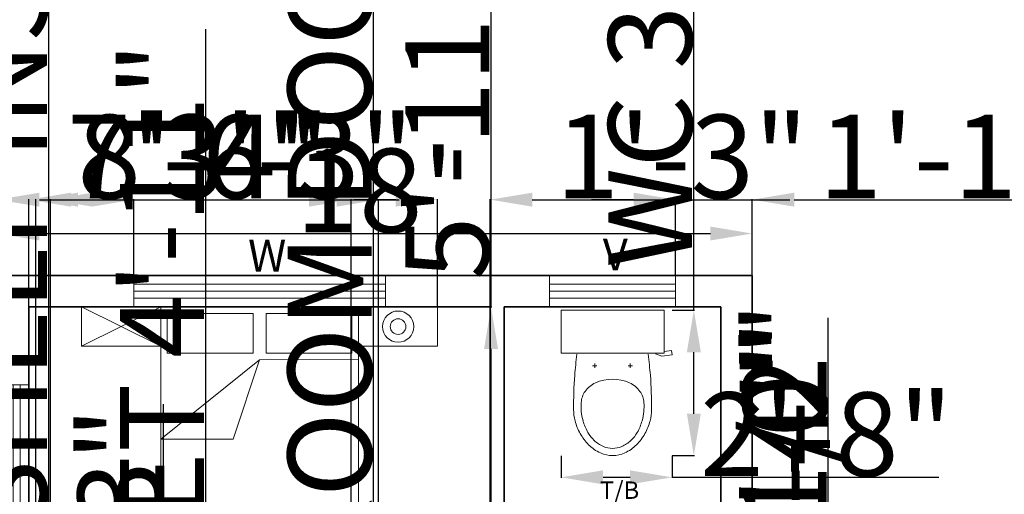
# Model space of a CAD drawing. Units: inches. Extents: x 2236 to 2927, y 1577 to 2452.
# Tile 7 of 9: x 2413 to 2695, y 2021 to 2157. Entities that reach past the tile are written whole.
import ezdxf

# ---------------------------------------------------------------- set-up
doc = ezdxf.new("R2010")
doc.units = ezdxf.units.IN
for name, color, linetype, lineweight in [('A-ANNO-DIMS', 2, 'Continuous', 18), ('A-ANNO-TEXT', 7, 'Continuous', 18), ('A-AREA-IDEN', 7, 'Continuous', 18), ('A-FLOR-FIXT', 9, 'Continuous', 18), ('A-FURN', 8, 'Continuous', 18), ('Wall', 7, 'Continuous', 35), ('Windows', 162, 'Continuous', 18)]:
    doc.layers.add(name, color=color, linetype=linetype, lineweight=lineweight)
doc.styles.get("Standard").update_dxf_attribs({"font": 'arial.ttf'})
doc.dimstyles.get("Standard").update_dxf_attribs({"dimtxt": 24, "dimasz": 12, "dimexe": 0.18, "dimexo": 0.0625, "dimgap": 0.09, "dimtad": 1, "dimdec": 1, "dimzin": 0, "dimdsep": 46, "dimlunit": 4, "dimtxsty": 'Standard', "dimcen": 0.09, "dimadec": 0, "dimazin": 0, "dimtfac": 1, "dimtdec": 1, "dimtofl": 0, "dimtmove": 0, "dimatfit": 3, "dimfxl": 1, "dimtolj": 1, "dimtzin": 0, "dimarcsym": 0})

# ---------------------------------------------------------------- blocks, each defined once
blk = doc.blocks.new('MAT-P13')
for p, q in [((-1.3496, 0), (-0.75, 0)), ((-1.3496, 0), (-1.3496, -0.2983)), ((-1.3496, -0.2983), (-0.75, 0)), ((-1.3496, 0), (-0.75, -0.2983)), ((-0.75, 0), (0.75, 0)), ((-0.75, 0), (-0.75, -1.9)), ((0.75, 0), (0.75, -1.9)), ((0.75, 0), (1.3496, 0)), ((1.3496, 0), (1.3496, -0.2983)), ((-0.7, -0.05), (-0.7, -0.35)), ((-0.7, -0.05), (-0.05, -0.05)), ((-0.05, -0.35), (-0.05, -0.05)), ((0.05, -0.05), (0.7, -0.05)), ((0.05, -0.35), (0.05, -0.05)), ((0.7, -0.05), (0.7, -0.35)), ((-0.75, -0.2983), (-1.3496, -0.2983)), ((1.3496, -0.2983), (0.75, -0.2983)), ((-0.7, -0.35), (-0.05, -0.35)), ((0.05, -0.35), (0.7, -0.35)), ((-0.75, -1.0034), (0, -0.4)), ((0, -0.4), (-0.75, -1.0034)), ((0, -0.4), (-0.2, -1.0034)), ((0, -0.4), (0.75, -0.398)), ((-0.75, -1.0034), (-0.2, -1.0034)), ((0.75, -1.9), (-0.75, -1.9))]:
    blk.add_line(p, q)
for radius in [0.1186, 0.0593]:
    blk.add_circle((1.0498, -0.1491), radius)
blk = doc.blocks.new('toilet-1')
at = {"color": 0, "linetype": 'ByBlock'}
for p, q in [((-0.23, -0.02), (-0.23, -0.2116)), ((0.23, -0.02), (-0.23, -0.02)), ((0.23, -0.02), (0.23, -0.2116)), ((-0.23, -0.2116), (0.23, -0.2116)), ((0.1917, -0.2144), (0.2206, -0.225)), ((0.2206, -0.225), (0.266, -0.2187)), ((0.2633, -0.1997), (0.23, -0.2044)), ((0.266, -0.2187), (0.2633, -0.1997)), ((-0.0793, -0.2587), (-0.0793, -0.2778)), ((0.0794, -0.2587), (0.0794, -0.2778)), ((-0.0889, -0.2683), (-0.0697, -0.2683)), ((0.0889, -0.2683), (0.0698, -0.2683)), ((0, -0.6382), (0, -0.6382))]:
    blk.add_line(p, q, dxfattribs=at)
for centre, radius, start, end in [((3.5272, -0.6239), 3.7093, 173.6925, 175.1593), ((-3.527, -0.624), 3.7093, 4.8413, 6.3171), ((1.7368, -0.4519), 1.9109, 175.7698, 180.3758), ((-0.0312, -0.4465), 0.1114, 113.8997, 145.1485), ((0, -0.5169), 0.1884, 66.0939, 113.9061), ((0.0312, -0.4465), 0.1114, 34.8515, 66.1003), ((-1.7366, -0.4519), 1.9109, 359.6242, 4.2302), ((-0.0408, -0.4398), 0.0996, 145.1497, 175.881), ((0.0409, -0.4398), 0.0996, 4.119, 34.8503), ((0.0981, -0.4497), 0.2389, 175.8862, 195.5931), ((-0.098, -0.4497), 0.2389, 344.4069, 4.1138), ((0.0353, -0.463), 0.2093, 180.3747, 194.3375), ((-0.0351, -0.463), 0.2093, 345.6614, 359.6243), ((0.055, -0.458), 0.2297, 194.3353, 209.622), ((0.0961, -0.4503), 0.2369, 195.5969, 209.3771), ((-0.096, -0.4503), 0.2369, 330.6229, 344.4031), ((-0.0548, -0.458), 0.2297, 330.3788, 345.6655), ((0.0647, -0.4524), 0.2409, 209.6273, 224.5489), ((0.0232, -0.4913), 0.1532, 209.3871, 226.5438), ((-0.0231, -0.4913), 0.1532, 313.4562, 330.6129), ((-0.0645, -0.4524), 0.2409, 315.4504, 330.372), ((0.0152, -0.4997), 0.1416, 226.5501, 246.5527), ((-0.0151, -0.4997), 0.1416, 293.4473, 313.4499), ((0.0178, -0.4986), 0.1751, 224.552, 245.714), ((0.0004, -0.538), 0.132, 245.5845, 269.8782), ((0, -0.5347), 0.1034, 246.5493, 270.0042), ((0, -0.5347), 0.1034, 269.9958, 293.4507), ((-0.0002, -0.538), 0.132, 270.1216, 294.4153), ((-0.0176, -0.4986), 0.1751, 294.2865, 315.4485)]:
    blk.add_arc(centre, radius, start, end, dxfattribs=at)
blk = doc.blocks.new('*D9')
at = {"layer": 'A-ANNO-DIMS', "color": 0, "lineweight": -2, "transparency": 16777216}
for p, q in [((2406.85, 2084.14), (2406.85, 2096.31)), ((2418.85, 2096.13), (2610.85, 2096.13)), ((2622.85, 2084.14), (2622.85, 2096.31))]:
    blk.add_line(p, q, dxfattribs=at)
at = {"layer": 'A-ANNO-DIMS', "color": 0, "transparency": 16777216}
for points in [[(2418.85, 2098.13), (2418.85, 2094.13), (2406.85, 2096.13)], [(2610.85, 2098.13), (2610.85, 2094.13), (2622.85, 2096.13)]]:
    blk.add_solid(points, dxfattribs=at)
at = {"layer": 'Defpoints', "color": 0, "transparency": 16777216}
for p in [(2622.85, 2096.13), (2406.85, 2084.08), (2622.85, 2084.08)]:
    blk.add_point(p, dxfattribs=at)
at = {"layer": 'A-ANNO-DIMS', "color": 0, "transparency": 16777216, "insert": (2514.85, 2108.47), "char_height": 24, "attachment_point": 5}
blk.add_mtext("\\A1;18'", dxfattribs=at)
blk = doc.blocks.new('WIN-72IN')
for p, q in [((0, 6.5), (72, 6.5)), ((0, 4.5), (72, 4.5)), ((0, 2.5), (72, 2.5))]:
    blk.add_line(p, q)
blk.add_lwpolyline([(0, 9), (72, 9), (72, 0), (0, 0)], close=True)
blk = doc.blocks.new('WIN-36IN')
for p, q in [((2.5, 0), (2.5, 36)), ((4.5, 0), (4.5, 36)), ((6.5, 0), (6.5, 36))]:
    blk.add_line(p, q)
blk.add_lwpolyline([(0, 0), (0, 36), (9, 36), (9, 0)], close=True)
blk = doc.blocks.new('*D16')
at = {"layer": 'A-ANNO-DIMS', "color": 0, "lineweight": -2, "transparency": 16777216}
for p, q in [((2421.54, 1988.01), (2421.54, 2451.93)), ((2421.05, 1976.01), (2421.72, 1976.01)), ((2421.05, 1972.34), (2421.72, 1972.34)), ((2421.54, 1960.34), (2421.54, 1948.34))]:
    blk.add_line(p, q, dxfattribs=at)
at = {"layer": 'A-ANNO-DIMS', "color": 0, "transparency": 16777216}
for points in [[(2419.54, 1988.01), (2423.54, 1988.01), (2421.54, 1976.01)], [(2419.54, 1960.34), (2423.54, 1960.34), (2421.54, 1972.34)]]:
    blk.add_solid(points, dxfattribs=at)
at = {"layer": 'Defpoints', "color": 0, "transparency": 16777216}
for p in [(2420.99, 1976.01), (2421.54, 1976.01), (2420.99, 1972.34)]:
    blk.add_point(p, dxfattribs=at)
at = {"layer": 'A-ANNO-DIMS', "color": 0, "transparency": 16777216, "insert": (2409.03, 2225.97), "char_height": 24, "attachment_point": 5, "rotation": 90}
blk.add_mtext('\\A1;SHELF INSERT 0\'-3 1/2" TYP.', dxfattribs=at)
blk = doc.blocks.new('*D18')
at = {"layer": 'A-ANNO-DIMS', "color": 0, "lineweight": -2, "transparency": 16777216}
for p, q in [((2396.05, 1834.44), (2396.05, 2191.28)), ((2406.79, 1834.44), (2395.87, 1834.44)), ((2396.05, 1774.44), (2396.05, 1822.44)), ((2406.79, 1762.44), (2395.87, 1762.44))]:
    blk.add_line(p, q, dxfattribs=at)
at = {"layer": 'A-ANNO-DIMS', "color": 0, "transparency": 16777216}
for points in [[(2394.05, 1822.44), (2398.05, 1822.44), (2396.05, 1834.44)], [(2394.05, 1774.44), (2398.05, 1774.44), (2396.05, 1762.44)]]:
    blk.add_solid(points, dxfattribs=at)
at = {"layer": 'Defpoints', "color": 0, "transparency": 16777216}
for p in [(2396.05, 1834.44), (2406.85, 1834.44), (2406.85, 1762.44)]:
    blk.add_point(p, dxfattribs=at)
at = {"layer": 'A-ANNO-DIMS', "color": 0, "transparency": 16777216, "insert": (2383.54, 2018.86), "char_height": 24, "attachment_point": 5, "rotation": 90}
blk.add_mtext('\\A1;WINDOW W 6\'-0" TYP.', dxfattribs=at)
blk = doc.blocks.new('*D20')
at = {"layer": 'A-ANNO-DIMS', "color": 0, "lineweight": -2, "transparency": 16777216}
for p, q in [((2401.45, 1929.71), (2401.45, 2363.75)), ((2406.79, 1929.71), (2401.27, 1929.71)), ((2401.45, 1905.71), (2401.45, 1917.71)), ((2406.79, 1893.71), (2401.27, 1893.71))]:
    blk.add_line(p, q, dxfattribs=at)
at = {"layer": 'A-ANNO-DIMS', "color": 0, "transparency": 16777216}
for points in [[(2399.45, 1917.71), (2403.45, 1917.71), (2401.45, 1929.71)], [(2399.45, 1905.71), (2403.45, 1905.71), (2401.45, 1893.71)]]:
    blk.add_solid(points, dxfattribs=at)
at = {"layer": 'Defpoints', "color": 0, "transparency": 16777216}
for p in [(2401.45, 1929.71), (2406.85, 1929.71), (2406.85, 1893.71)]:
    blk.add_point(p, dxfattribs=at)
at = {"layer": 'A-ANNO-DIMS', "color": 0, "transparency": 16777216, "insert": (2388.93, 2152.73), "char_height": 24, "attachment_point": 5, "rotation": 90}
blk.add_mtext('\\A1;SMALL WINDOW 3\'-0" TYP.', dxfattribs=at)
blk = doc.blocks.new('*D22')
at = {"layer": 'A-ANNO-DIMS', "color": 0, "lineweight": -2, "transparency": 16777216}
for p, q in [((2514.42, 1977.96), (2514.42, 2358.7)), ((2518.53, 1977.96), (2514.24, 1977.96)), ((2514.42, 1962.08), (2514.42, 1965.96)), ((2518.53, 1950.08), (2514.24, 1950.08))]:
    blk.add_line(p, q, dxfattribs=at)
at = {"layer": 'A-ANNO-DIMS', "color": 0, "transparency": 16777216}
for points in [[(2512.42, 1965.96), (2516.42, 1965.96), (2514.42, 1977.96)], [(2512.42, 1962.08), (2516.42, 1962.08), (2514.42, 1950.08)]]:
    blk.add_solid(points, dxfattribs=at)
at = {"layer": 'Defpoints', "color": 0, "transparency": 16777216}
for p in [(2514.42, 1977.96), (2518.6, 1977.96), (2518.6, 1950.08)]:
    blk.add_point(p, dxfattribs=at)
at = {"layer": 'A-ANNO-DIMS', "color": 0, "transparency": 16777216, "insert": (2501.91, 2174.33), "char_height": 24, "attachment_point": 5, "rotation": 90}
blk.add_mtext('\\A1;ROOM DOOR 2\'-4" TYP.', dxfattribs=at)
blk = doc.blocks.new('*D28')
at = {"layer": 'A-ANNO-DIMS', "color": 0, "lineweight": -2, "transparency": 16777216}
for p, q in [((2430.9, 2003.29), (2430.9, 1987.89)), ((2532.8, 2003.29), (2532.8, 1987.89)), ((2442.9, 1988.07), (2520.8, 1988.07)), ((2532.8, 1988.07), (2818.23, 1988.07))]:
    blk.add_line(p, q, dxfattribs=at)
at = {"layer": 'A-ANNO-DIMS', "color": 0, "transparency": 16777216}
for points in [[(2442.9, 1990.07), (2442.9, 1986.07), (2430.9, 1988.07)], [(2520.8, 1990.07), (2520.8, 1986.07), (2532.8, 1988.07)]]:
    blk.add_solid(points, dxfattribs=at)
at = {"layer": 'Defpoints', "color": 0, "transparency": 16777216}
for p in [(2430.9, 2003.35), (2532.8, 2003.35), (2532.8, 1988.07)]:
    blk.add_point(p, dxfattribs=at)
at = {"layer": 'A-ANNO-DIMS', "color": 0, "transparency": 16777216, "insert": (2681.51, 2000.57), "char_height": 24, "attachment_point": 5}
blk.add_mtext('\\A1;BED GROUP 8\'-6"', dxfattribs=at)
blk = doc.blocks.new('*D29')
at = {"layer": 'A-ANNO-DIMS', "color": 0, "lineweight": -2, "transparency": 16777216}
for p, q in [((2548.08, 2075.08), (2548.08, 2225.62)), ((2532.86, 2075.08), (2548.26, 2075.08)), ((2548.08, 2015.35), (2548.08, 2063.08)), ((2532.86, 2003.35), (2548.26, 2003.35))]:
    blk.add_line(p, q, dxfattribs=at)
at = {"layer": 'A-ANNO-DIMS', "color": 0, "transparency": 16777216}
for points in [[(2546.08, 2063.08), (2550.08, 2063.08), (2548.08, 2075.08)], [(2546.08, 2015.35), (2550.08, 2015.35), (2548.08, 2003.35)]]:
    blk.add_solid(points, dxfattribs=at)
at = {"layer": 'Defpoints', "color": 0, "transparency": 16777216}
for p in [(2532.8, 2075.08), (2548.08, 2075.08), (2532.8, 2003.35)]:
    blk.add_point(p, dxfattribs=at)
at = {"layer": 'A-ANNO-DIMS', "color": 0, "transparency": 16777216, "insert": (2535.58, 2156.35), "char_height": 24, "attachment_point": 5, "rotation": 90}
blk.add_mtext('\\A1;5\'-11 1/2"', dxfattribs=at)
blk = doc.blocks.new('*D30')
at = {"layer": 'A-ANNO-DIMS', "color": 0, "lineweight": -2, "transparency": 16777216}
for p, q in [((2606.12, 2074.13), (2606.12, 2272.19)), ((2599.94, 2074.13), (2606.3, 2074.13)), ((2606.12, 2044.51), (2606.12, 2062.13)), ((2599.94, 2032.51), (2606.3, 2032.51))]:
    blk.add_line(p, q, dxfattribs=at)
at = {"layer": 'A-ANNO-DIMS', "color": 0, "transparency": 16777216}
for points in [[(2604.12, 2062.13), (2608.12, 2062.13), (2606.12, 2074.13)], [(2604.12, 2044.51), (2608.12, 2044.51), (2606.12, 2032.51)]]:
    blk.add_solid(points, dxfattribs=at)
at = {"layer": 'Defpoints', "color": 0, "transparency": 16777216}
for p in [(2599.88, 2074.13), (2606.12, 2074.13), (2599.88, 2032.51)]:
    blk.add_point(p, dxfattribs=at)
at = {"layer": 'A-ANNO-DIMS', "color": 0, "transparency": 16777216, "insert": (2593.61, 2179.16), "char_height": 24, "attachment_point": 5, "rotation": 90}
blk.add_mtext('\\A1;WC 3\'-5 1/2"', dxfattribs=at)
blk = doc.blocks.new('*D31')
at = {"layer": 'A-ANNO-DIMS', "color": 0, "lineweight": -2, "transparency": 16777216}
for p, q in [((2568.12, 2032.45), (2568.12, 2026.09)), ((2599.88, 2032.45), (2599.88, 2026.09)), ((2580.12, 2026.27), (2587.88, 2026.27)), ((2599.88, 2026.27), (2676.27, 2026.27))]:
    blk.add_line(p, q, dxfattribs=at)
at = {"layer": 'A-ANNO-DIMS', "color": 0, "transparency": 16777216}
for points in [[(2580.12, 2028.27), (2580.12, 2024.27), (2568.12, 2026.27)], [(2587.88, 2028.27), (2587.88, 2024.27), (2599.88, 2026.27)]]:
    blk.add_solid(points, dxfattribs=at)
at = {"layer": 'Defpoints', "color": 0, "transparency": 16777216}
for p in [(2568.12, 2032.51), (2599.88, 2032.51), (2599.88, 2026.27)]:
    blk.add_point(p, dxfattribs=at)
at = {"layer": 'A-ANNO-DIMS', "color": 0, "transparency": 16777216, "insert": (2644.07, 2038.61), "char_height": 24, "attachment_point": 5}
blk.add_mtext('\\A1;2\'-8"', dxfattribs=at)
blk = doc.blocks.new('*D36')
at = {"layer": 'A-ANNO-DIMS', "color": 0, "lineweight": -2, "transparency": 16777216}
for p, q in [((2454.3, 1796.23), (2454.3, 2047.2)), ((2444.91, 1796.23), (2454.48, 1796.23)), ((2454.3, 1745.23), (2454.3, 1784.23)), ((2444.91, 1733.23), (2454.48, 1733.23))]:
    blk.add_line(p, q, dxfattribs=at)
at = {"layer": 'A-ANNO-DIMS', "color": 0, "transparency": 16777216}
for points in [[(2452.3, 1784.23), (2456.3, 1784.23), (2454.3, 1796.23)], [(2452.3, 1745.23), (2456.3, 1745.23), (2454.3, 1733.23)]]:
    blk.add_solid(points, dxfattribs=at)
at = {"layer": 'Defpoints', "color": 0, "transparency": 16777216}
for p in [(2444.85, 1796.23), (2454.3, 1796.23), (2444.85, 1733.23)]:
    blk.add_point(p, dxfattribs=at)
at = {"layer": 'A-ANNO-DIMS', "color": 0, "transparency": 16777216, "insert": (2441.79, 1927.72), "char_height": 24, "attachment_point": 5, "rotation": 90}
blk.add_mtext('\\A1;SINK UNIT 5\'-3"', dxfattribs=at)
blk = doc.blocks.new('*D38')
at = {"layer": 'A-ANNO-DIMS', "color": 0, "lineweight": -2, "transparency": 16777216}
for p, q in [((2466.44, 1860.06), (2466.44, 2154.67)), ((2457.67, 1860.06), (2466.62, 1860.06)), ((2466.44, 1813.15), (2466.44, 1848.06)), ((2457.67, 1801.15), (2466.62, 1801.15))]:
    blk.add_line(p, q, dxfattribs=at)
at = {"layer": 'A-ANNO-DIMS', "color": 0, "transparency": 16777216}
for points in [[(2464.44, 1848.06), (2468.44, 1848.06), (2466.44, 1860.06)], [(2464.44, 1813.15), (2468.44, 1813.15), (2466.44, 1801.15)]]:
    blk.add_solid(points, dxfattribs=at)
at = {"layer": 'Defpoints', "color": 0, "transparency": 16777216}
for p in [(2457.61, 1860.06), (2466.44, 1860.06), (2457.61, 1801.15)]:
    blk.add_point(p, dxfattribs=at)
at = {"layer": 'A-ANNO-DIMS', "color": 0, "transparency": 16777216, "insert": (2453.94, 2013.36), "char_height": 24, "attachment_point": 5, "rotation": 90}
blk.add_mtext('\\A1;DINING SET 4\'-11"', dxfattribs=at)
blk = doc.blocks.new('*D40')
at = {"layer": 'A-ANNO-DIMS', "color": 0, "lineweight": -2, "transparency": 16777216}
for p, q in [((2406.85, 2084.14), (2406.85, 2106.01)), ((2418.85, 2105.83), (2433.85, 2105.83)), ((2445.85, 2084.14), (2445.85, 2106.01)), ((2445.85, 2105.83), (2521.81, 2105.83))]:
    blk.add_line(p, q, dxfattribs=at)
at = {"layer": 'A-ANNO-DIMS', "color": 0, "transparency": 16777216}
for points in [[(2418.85, 2107.83), (2418.85, 2103.83), (2406.85, 2105.83)], [(2433.85, 2107.83), (2433.85, 2103.83), (2445.85, 2105.83)]]:
    blk.add_solid(points, dxfattribs=at)
at = {"layer": 'Defpoints', "color": 0, "transparency": 16777216}
for p in [(2445.85, 2105.83), (2406.85, 2084.08), (2445.85, 2084.08)]:
    blk.add_point(p, dxfattribs=at)
at = {"layer": 'A-ANNO-DIMS', "color": 0, "transparency": 16777216, "insert": (2489.83, 2118.18), "char_height": 24, "attachment_point": 5}
blk.add_mtext('\\A1;3\'-3"', dxfattribs=at)
blk = doc.blocks.new('*D41')
at = {"layer": 'A-ANNO-DIMS', "color": 0, "lineweight": -2, "transparency": 16777216}
for p, q in [((2588.85, 2105.83), (2576.85, 2105.83)), ((2600.85, 2084.14), (2600.85, 2106.01)), ((2622.85, 2084.14), (2622.85, 2106.01)), ((2634.85, 2105.83), (2727.21, 2105.83))]:
    blk.add_line(p, q, dxfattribs=at)
at = {"layer": 'A-ANNO-DIMS', "color": 0, "transparency": 16777216}
for points in [[(2588.85, 2107.83), (2588.85, 2103.83), (2600.85, 2105.83)], [(2634.85, 2107.83), (2634.85, 2103.83), (2622.85, 2105.83)]]:
    blk.add_solid(points, dxfattribs=at)
at = {"layer": 'Defpoints', "color": 0, "transparency": 16777216}
for p in [(2622.85, 2105.83), (2600.85, 2084.08), (2622.85, 2084.08)]:
    blk.add_point(p, dxfattribs=at)
at = {"layer": 'A-ANNO-DIMS', "color": 0, "transparency": 16777216, "insert": (2687.03, 2118.17), "char_height": 24, "attachment_point": 5}
blk.add_mtext('\\A1;1\'-10"', dxfattribs=at)
blk = doc.blocks.new('*D52')
at = {"layer": 'A-ANNO-DIMS', "color": 0, "lineweight": -2, "transparency": 16777216}
for p, q in [((2415.85, 1979.14), (2415.85, 2106.01)), ((2427.85, 2105.83), (2503.88, 2105.83)), ((2515.88, 1979.14), (2515.88, 2106.01))]:
    blk.add_line(p, q, dxfattribs=at)
at = {"layer": 'A-ANNO-DIMS', "color": 0, "transparency": 16777216}
for points in [[(2427.85, 2107.83), (2427.85, 2103.83), (2415.85, 2105.83)], [(2503.88, 2107.83), (2503.88, 2103.83), (2515.88, 2105.83)]]:
    blk.add_solid(points, dxfattribs=at)
at = {"layer": 'Defpoints', "color": 0, "transparency": 16777216}
for p in [(2515.88, 2105.83), (2415.85, 1979.08), (2515.88, 1979.08)]:
    blk.add_point(p, dxfattribs=at)
at = {"layer": 'A-ANNO-DIMS', "color": 0, "transparency": 16777216, "insert": (2465.87, 2118.17), "char_height": 24, "attachment_point": 5}
blk.add_mtext('\\A1;8\'-4"', dxfattribs=at)
blk = doc.blocks.new('*D53')
at = {"layer": 'A-ANNO-DIMS', "color": 0, "lineweight": -2, "transparency": 16777216}
for p, q in [((2644.6, 1991.08), (2644.6, 2067.46)), ((2515.94, 1979.08), (2644.78, 1979.08)), ((2515.94, 1955.08), (2644.78, 1955.08)), ((2644.6, 1943.08), (2644.6, 1931.08))]:
    blk.add_line(p, q, dxfattribs=at)
at = {"layer": 'A-ANNO-DIMS', "color": 0, "transparency": 16777216}
for points in [[(2642.6, 1991.08), (2646.6, 1991.08), (2644.6, 1979.08)], [(2642.6, 1943.08), (2646.6, 1943.08), (2644.6, 1955.08)]]:
    blk.add_solid(points, dxfattribs=at)
at = {"layer": 'Defpoints', "color": 0, "transparency": 16777216}
for p in [(2515.88, 1979.08), (2644.6, 1979.08), (2515.88, 1955.08)]:
    blk.add_point(p, dxfattribs=at)
at = {"layer": 'A-ANNO-DIMS', "color": 0, "transparency": 16777216, "insert": (2632.25, 2035.27), "char_height": 24, "attachment_point": 5, "rotation": 90}
blk.add_mtext('\\A1;2\'-0"', dxfattribs=at)
blk = doc.blocks.new('*D61')
at = {"layer": 'A-ANNO-DIMS', "color": 0, "lineweight": -2, "transparency": 16777216}
for p, q in [((2403.85, 2105.83), (2327.87, 2105.83)), ((2415.85, 1869.14), (2415.85, 2106.01)), ((2422.01, 1844.91), (2422.01, 2106.01)), ((2434.01, 2105.83), (2446.01, 2105.83))]:
    blk.add_line(p, q, dxfattribs=at)
at = {"layer": 'A-ANNO-DIMS', "color": 0, "transparency": 16777216}
for points in [[(2403.85, 2107.83), (2403.85, 2103.83), (2415.85, 2105.83)], [(2434.01, 2107.83), (2434.01, 2103.83), (2422.01, 2105.83)]]:
    blk.add_solid(points, dxfattribs=at)
at = {"layer": 'Defpoints', "color": 0, "transparency": 16777216}
for p in [(2415.85, 2105.83), (2415.85, 1869.08), (2422.01, 1844.84)]:
    blk.add_point(p, dxfattribs=at)
at = {"layer": 'A-ANNO-DIMS', "color": 0, "transparency": 16777216, "insert": (2359.86, 2118.17), "char_height": 24, "attachment_point": 5}
blk.add_mtext('\\A1;0\'-6"', dxfattribs=at)
blk = doc.blocks.new('*D62')
at = {"layer": 'A-ANNO-DIMS', "color": 0, "lineweight": -2, "transparency": 16777216}
for p, q in [((2417.85, 1972.4), (2417.85, 2106.01)), ((2429.85, 2105.83), (2496.01, 2105.83)), ((2508.01, 1972.4), (2508.01, 2106.01))]:
    blk.add_line(p, q, dxfattribs=at)
at = {"layer": 'A-ANNO-DIMS', "color": 0, "transparency": 16777216}
for points in [[(2429.85, 2107.83), (2429.85, 2103.83), (2417.85, 2105.83)], [(2496.01, 2107.83), (2496.01, 2103.83), (2508.01, 2105.83)]]:
    blk.add_solid(points, dxfattribs=at)
at = {"layer": 'Defpoints', "color": 0, "transparency": 16777216}
for p in [(2508.01, 2105.83), (2417.85, 1972.34), (2508.01, 1972.34)]:
    blk.add_point(p, dxfattribs=at)
at = {"layer": 'A-ANNO-DIMS', "color": 0, "transparency": 16777216, "insert": (2462.93, 2118.17), "char_height": 24, "attachment_point": 5}
blk.add_mtext('\\A1;7\'-6"', dxfattribs=at)
blk = doc.blocks.new('*D63')
at = {"layer": 'A-ANNO-DIMS', "color": 0, "lineweight": -2, "transparency": 16777216}
for p, q in [((2644.6, 1984.34), (2644.6, 2058.06)), ((2511.22, 1972.34), (2644.78, 1972.34)), ((2511.22, 1956.39), (2644.78, 1956.39)), ((2644.6, 1944.39), (2644.6, 1932.39))]:
    blk.add_line(p, q, dxfattribs=at)
at = {"layer": 'A-ANNO-DIMS', "color": 0, "transparency": 16777216}
for points in [[(2642.6, 1984.34), (2646.6, 1984.34), (2644.6, 1972.34)], [(2642.6, 1944.39), (2646.6, 1944.39), (2644.6, 1956.39)]]:
    blk.add_solid(points, dxfattribs=at)
at = {"layer": 'Defpoints', "color": 0, "transparency": 16777216}
for p in [(2511.16, 1972.34), (2644.6, 1972.34), (2511.16, 1956.39)]:
    blk.add_point(p, dxfattribs=at)
at = {"layer": 'A-ANNO-DIMS', "color": 0, "transparency": 16777216, "insert": (2632.46, 2027.2), "char_height": 24, "attachment_point": 5, "rotation": 90}
blk.add_mtext('\\A1;1\'-4"', dxfattribs=at)
blk = doc.blocks.new('*D65')
at = {"layer": 'A-ANNO-DIMS', "color": 0, "lineweight": -2, "transparency": 16777216}
for p, q in [((2644.6, 1940.08), (2644.6, 2071.98)), ((2580.91, 1928.08), (2644.78, 1928.08)), ((2569.48, 1919.34), (2644.78, 1919.34)), ((2644.6, 1907.34), (2644.6, 1895.34))]:
    blk.add_line(p, q, dxfattribs=at)
at = {"layer": 'A-ANNO-DIMS', "color": 0, "transparency": 16777216}
for points in [[(2642.6, 1940.08), (2646.6, 1940.08), (2644.6, 1928.08)], [(2642.6, 1907.34), (2646.6, 1907.34), (2644.6, 1919.34)]]:
    blk.add_solid(points, dxfattribs=at)
at = {"layer": 'Defpoints', "color": 0, "transparency": 16777216}
for p in [(2580.85, 1928.08), (2644.6, 1928.08), (2569.42, 1919.34)]:
    blk.add_point(p, dxfattribs=at)
at = {"layer": 'A-ANNO-DIMS', "color": 0, "transparency": 16777216, "insert": (2632.1, 2012.03), "char_height": 24, "attachment_point": 5, "rotation": 90}
blk.add_mtext('\\A1;0\'-8 1/2"', dxfattribs=at)
blk = doc.blocks.new('*D66')
at = {"layer": 'A-ANNO-DIMS', "color": 0, "lineweight": -2, "transparency": 16777216}
for p, q in [((2520.8, 2105.83), (2508.8, 2105.83)), ((2532.8, 2075.14), (2532.8, 2106.01)), ((2547.85, 2075.14), (2547.85, 2106.01)), ((2559.85, 2105.83), (2633.57, 2105.83))]:
    blk.add_line(p, q, dxfattribs=at)
at = {"layer": 'A-ANNO-DIMS', "color": 0, "transparency": 16777216}
for points in [[(2520.8, 2107.83), (2520.8, 2103.83), (2532.8, 2105.83)], [(2559.85, 2107.83), (2559.85, 2103.83), (2547.85, 2105.83)]]:
    blk.add_solid(points, dxfattribs=at)
at = {"layer": 'Defpoints', "color": 0, "transparency": 16777216}
for p in [(2547.85, 2105.83), (2532.8, 2075.08), (2547.85, 2075.08)]:
    blk.add_point(p, dxfattribs=at)
at = {"layer": 'A-ANNO-DIMS', "color": 0, "transparency": 16777216, "insert": (2602.71, 2118.18), "char_height": 24, "attachment_point": 5}
blk.add_mtext('\\A1;1\'-3"', dxfattribs=at)

msp = doc.modelspace()

# ---------------------------------------------------------------- linework, layer by layer
at = {"layer": 'Wall'}
for p, q in [((2406.85, 2084.08), (2622.85, 2084.08)), ((2622.85, 2084.08), (2622.85, 1724.08)), ((2415.85, 2075.08), (2547.85, 2075.08)), ((2415.85, 2075.08), (2415.85, 1955.08)), ((2547.85, 2075.08), (2547.85, 1955.08)), ((2551.85, 2075.08), (2551.85, 1991.08)), ((2551.85, 2075.08), (2613.85, 2075.08)), ((2613.85, 2075.08), (2613.85, 1991.08))]:
    msp.add_line(p, q, dxfattribs=at)

# ---------------------------------------------------------------- block references
at = {"layer": 'A-FLOR-FIXT', "xscale": 64.02779084387056, "yscale": 64.02779084387056, "zscale": 64.02779084387056}
msp.add_blockref('toilet-1', (2582.85, 2075.41), dxfattribs=at)
at = {"layer": 'A-FURN', "xscale": 37.75073971806934, "yscale": 37.75073971806934, "zscale": 37.75073971806934}
msp.add_blockref('MAT-P13', (2481.85, 2075.08), dxfattribs=at)
at = {"layer": 'Windows'}
msp.add_blockref('WIN-72IN', (2445.85, 2075.08), dxfattribs=at)
for name, p, rotation in [('WIN-36IN', (2600.85, 2075.08), 89.99999999999923), ('WIN-72IN', (2415.85, 1980.78), 90.00000000000261)]:
    msp.add_blockref(name, p, dxfattribs=dict(at, rotation=rotation))

# ---------------------------------------------------------------- texts
at = {"layer": 'A-ANNO-TEXT'}
for s, p in [('W', (2478.55, 2085.21)), ('V', (2580.06, 2085.56))]:
    msp.add_text(s, height=9.12, dxfattribs=at).set_placement(p)
at = {"layer": 'A-AREA-IDEN', "insert": (2566.14, 2025.09), "char_height": 5, "attachment_point": 1}
msp.add_mtext_dynamic_manual_height_columns("\\pxqc;T/B\\P5'2''X7'", width=37.4353, gutter_width=12.5, heights=[0], dxfattribs=at)

# ---------------------------------------------------------------- dimensions: what is measured, and where the dimension line sits
at = {"layer": 'A-ANNO-DIMS'}
for base, p1, p2, text, picture, middle in [((2421.54, 1976.01), (2420.99, 1972.34), (2420.99, 1976.01), 'SHELF INSERT <> TYP.', '*D16', (2409.03, 2225.97)), ((2401.45, 1929.71), (2406.85, 1893.71), (2406.85, 1929.71), 'SMALL WINDOW <> TYP.', '*D20', (2388.93, 2152.73)), ((2514.42, 1977.96), (2518.6, 1950.08), (2518.6, 1977.96), 'ROOM DOOR <> TYP.', '*D22', (2501.91, 2174.33)), ((2606.12, 2074.13), (2599.88, 2032.51), (2599.88, 2074.13), 'WC <>', '*D30', (2593.61, 2179.16)), ((2396.05, 1834.44), (2406.85, 1762.44), (2406.85, 1834.44), 'WINDOW W <> TYP.', '*D18', (2383.54, 2018.86)), ((2466.44, 1860.06), (2457.61, 1801.15), (2457.61, 1860.06), 'DINING SET <>', '*D38', (2453.94, 2013.36)), ((2454.3, 1796.23), (2444.85, 1733.23), (2444.85, 1796.23), 'SINK UNIT <>', '*D36', (2441.79, 1927.72))]:
    dim = msp.add_linear_dim(base=base, p1=p1, p2=p2, angle=90, text=text, dimstyle='Standard', override={"dimdec": 1, "dimlfac": 1, "dimrnd": 0, "dimzin": 1, "dimdsep": 46, "dimlunit": 4, "dimfrac": 2}, dxfattribs=at)
    dim.commit()
    dim.dimension.update_dxf_attribs({"geometry": picture, "text_midpoint": middle})
for base, p1, p2, picture, middle in [((2548.08, 2075.08), (2532.8, 2003.35), (2532.8, 2075.08), '*D29', (2535.58, 2156.35)), ((2644.6, 1979.08), (2515.88, 1955.08), (2515.88, 1979.08), '*D53', (2632.25, 2035.27)), ((2644.6, 1928.08), (2569.42, 1919.34), (2580.85, 1928.08), '*D65', (2632.1, 2012.03)), ((2644.598, 1972.3393), (2511.1585, 1956.3877), (2511.1585, 1972.3393), '*D63', (2632.4589, 2027.1987))]:
    dim = msp.add_linear_dim(base=base, p1=p1, p2=p2, angle=90, dimstyle='Standard', override={"dimdec": 1, "dimlfac": 1, "dimrnd": 0, "dimzin": 1, "dimdsep": 46, "dimlunit": 4, "dimfrac": 2}, dxfattribs=at)
    dim.commit()
    dim.dimension.update_dxf_attribs({"geometry": picture, "text_midpoint": middle})
for base, p1, p2, override, picture, middle in [((2415.85, 2105.83), (2422.01, 1844.84), (2415.85, 1869.08), {"dimdec": 1, "dimlfac": 1, "dimrnd": 0, "dimzin": 1, "dimdsep": 46, "dimlunit": 4, "dimfrac": 2}, '*D61', (2359.86, 2118.17)), ((2445.85, 2105.83), (2406.85, 2084.08), (2445.85, 2084.08), {"dimdec": 1, "dimlfac": 1, "dimrnd": 0, "dimzin": 1, "dimdsep": 46, "dimlunit": 4, "dimfrac": 2}, '*D40', (2489.83, 2118.18)), ((2515.88, 2105.83), (2415.85, 1979.08), (2515.88, 1979.08), {"dimdec": 1, "dimlfac": 1, "dimrnd": 0, "dimzin": 1, "dimdsep": 46, "dimlunit": 4, "dimfrac": 2}, '*D52', (2465.87, 2118.17)), ((2508.01, 2105.83), (2417.85, 1972.34), (2508.01, 1972.34), {"dimdec": 1, "dimlfac": 1, "dimrnd": 0, "dimzin": 1, "dimdsep": 46, "dimlunit": 4, "dimfrac": 2}, '*D62', (2462.93, 2118.17)), ((2547.848, 2105.8263), (2532.7959, 2075.0763), (2547.848, 2075.0763), {"dimdec": 1, "dimlfac": 1, "dimrnd": 0, "dimzin": 1, "dimdsep": 46, "dimlunit": 4, "dimfrac": 2}, '*D66', (2602.7075, 2118.1782)), ((2622.85, 2105.83), (2600.85, 2084.08), (2622.85, 2084.08), {"dimdec": 1, "dimlfac": 1, "dimrnd": 0, "dimzin": 1, "dimdsep": 46, "dimlunit": 4, "dimfrac": 2}, '*D41', (2687.03, 2118.17)), ((2622.85, 2096.13), (2406.85, 2084.08), (2622.85, 2084.08), {"dimclrd": 0, "dimclre": 0, "dimclrt": 0}, '*D9', (2514.85, 2108.47)), ((2599.88, 2026.27), (2568.12, 2032.51), (2599.88, 2032.51), {"dimdec": 1, "dimlfac": 1, "dimrnd": 0, "dimzin": 1, "dimdsep": 46, "dimlunit": 4, "dimfrac": 2}, '*D31', (2644.07, 2038.61))]:
    dim = msp.add_linear_dim(base=base, p1=p1, p2=p2, dimstyle='Standard', override=override, dxfattribs=at)
    dim.commit()
    dim.dimension.update_dxf_attribs({"geometry": picture, "text_midpoint": middle})
dim = msp.add_linear_dim(base=(2532.8, 1988.07), p1=(2430.9, 2003.35), p2=(2532.8, 2003.35), text='BED GROUP <>', dimstyle='Standard', override={"dimdec": 1, "dimlfac": 1, "dimrnd": 0, "dimzin": 1, "dimdsep": 46, "dimlunit": 4, "dimfrac": 2}, dxfattribs=at)
dim.commit()
dim.dimension.update_dxf_attribs({"geometry": '*D28', "text_midpoint": (2681.51, 2000.57)})

doc.saveas('drawing.dxf')
